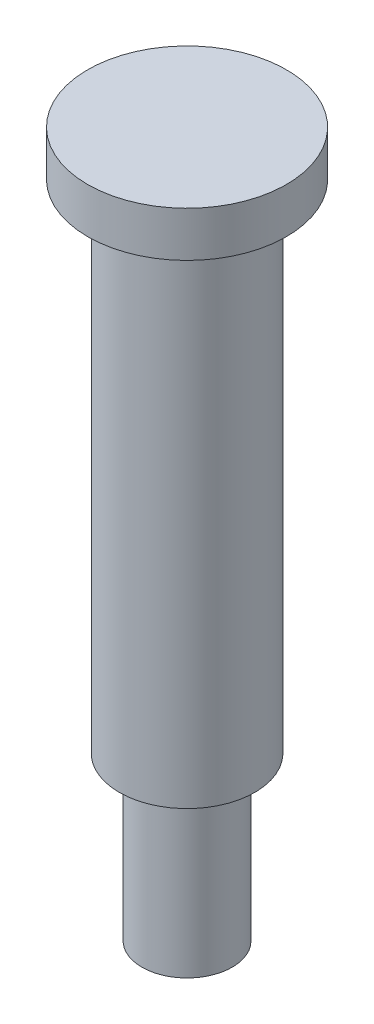
from build123d import *


with BuildPart() as part:
    # Pin Profile Sketch → Pin Body Revolve (revolve)
    with BuildSketch(Plane.XY, mode=Mode.PRIVATE) as pin_body_revolve_sk:
        Polygon((0, 0), (-11, 0), (-11, -5), (-7.5, -5), (-7.5, -60), (-5, -60), (-5, -78), (0, -78), align=None)
    revolve(pin_body_revolve_sk.sketch.rotate(Axis((0, 16.243243243, 0), (0, -1, 0)), 270), axis=Axis((0, 16.243243243, 0), (0, -1, 0)))


solid = part.part
